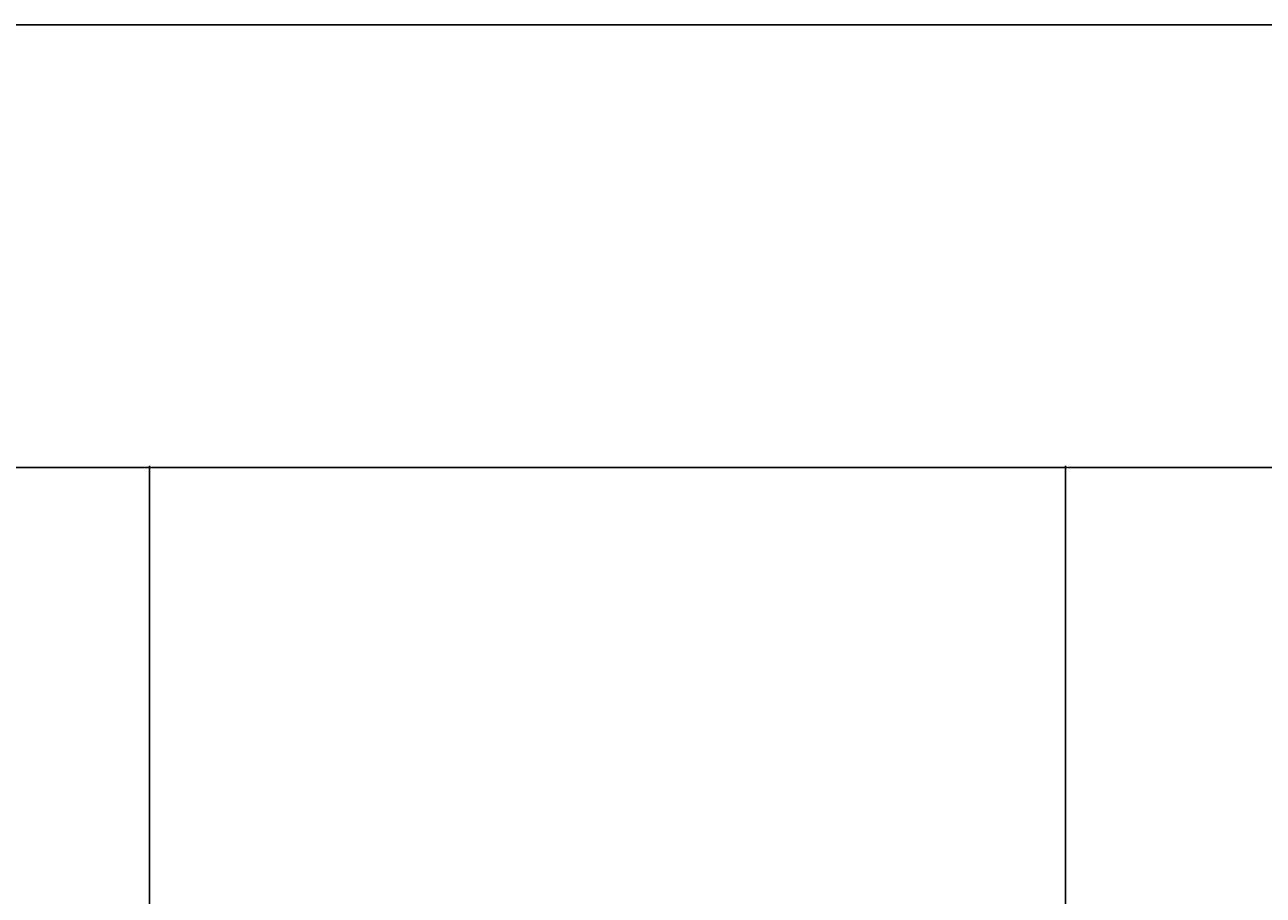
# Model space of a CAD drawing. Units: inches. Extents: x 1601 to 2297, y 1496 to 2631.
# Tile 45 of 57: x 1750 to 1891, y 2532 to 2631. Entities that reach past the tile are written whole.
import ezdxf

# ---------------------------------------------------------------- set-up
doc = ezdxf.new("R2010")
doc.units = ezdxf.units.IN
doc.layers.add('A-ANNO-DIMS', color=2, linetype='Continuous', lineweight=18)
doc.layers.add('A-ANNO-TTLB', color=7, linetype='Continuous', lineweight=25)
doc.styles.get("Standard").update_dxf_attribs({"font": 'arial.ttf'})
doc.dimstyles.get("Standard").update_dxf_attribs({"dimtxt": 0.18, "dimasz": 0.18, "dimexe": 0.18, "dimexo": 0.0625, "dimgap": 0.09, "dimtad": 0, "dimtih": 1, "dimtoh": 1, "dimdec": 4, "dimzin": 0, "dimdsep": 46, "dimtxsty": 'Standard', "dimcen": 0.09, "dimadec": 0, "dimazin": 0, "dimtfac": 1, "dimtdec": 4, "dimtofl": 0, "dimtmove": 0, "dimatfit": 3, "dimfxl": 1, "dimtolj": 1, "dimtzin": 0, "dimarcsym": 0})

# ---------------------------------------------------------------- blocks, each defined once
blk = doc.blocks.new('*D28')
at = {"layer": 'A-ANNO-DIMS', "color": 0, "lineweight": -2, "transparency": 16777216}
for p, q in [((1686.04, 2532.39), (1686.04, 2581.06)), ((1686.22, 2580.88), (1957.89, 2580.88)), ((2230.36, 2580.88), (1958.68, 2580.88)), ((2230.54, 2532.39), (2230.54, 2581.06))]:
    blk.add_line(p, q, dxfattribs=at)
at = {"layer": 'A-ANNO-DIMS', "color": 0, "transparency": 16777216}
for points in [[(1686.22, 2580.91), (1686.22, 2580.85), (1686.04, 2580.88)], [(2230.36, 2580.91), (2230.36, 2580.85), (2230.54, 2580.88)]]:
    blk.add_solid(points, dxfattribs=at)
at = {"layer": 'Defpoints', "color": 0, "transparency": 16777216}
for p in [(2230.54, 2580.88), (1686.04, 2532.33), (2230.54, 2532.33)]:
    blk.add_point(p, dxfattribs=at)
at = {"layer": 'A-ANNO-DIMS', "color": 0, "transparency": 16777216, "insert": (1958.29, 2580.88), "char_height": 0.18, "attachment_point": 5}
blk.add_mtext('\\A1;544.5', dxfattribs=at)
blk = doc.blocks.new('*D33')
at = {"layer": 'A-ANNO-DIMS', "color": 0, "lineweight": -2, "transparency": 16777216}
for p, q in [((1764.34, 2136.39), (1764.34, 2581.06)), ((1764.52, 2580.88), (1816.06, 2580.88)), ((1868.16, 2580.88), (1816.62, 2580.88)), ((1868.34, 2136.39), (1868.34, 2581.06))]:
    blk.add_line(p, q, dxfattribs=at)
at = {"layer": 'A-ANNO-DIMS', "color": 0, "transparency": 16777216}
for points in [[(1764.52, 2580.91), (1764.52, 2580.85), (1764.34, 2580.88)], [(1868.16, 2580.91), (1868.16, 2580.85), (1868.34, 2580.88)]]:
    blk.add_solid(points, dxfattribs=at)
at = {"layer": 'Defpoints', "color": 0, "transparency": 16777216}
for p in [(1868.34, 2580.88), (1764.34, 2136.33), (1868.34, 2136.33)]:
    blk.add_point(p, dxfattribs=at)
at = {"layer": 'A-ANNO-DIMS', "color": 0, "transparency": 16777216, "insert": (1816.34, 2580.88), "char_height": 0.18, "attachment_point": 5}
blk.add_mtext('\\A1;104', dxfattribs=at)

msp = doc.modelspace()

# ---------------------------------------------------------------- linework, layer by layer
at = {"layer": 'A-ANNO-TTLB'}
msp.add_lwpolyline([(1600.5933, 2631.1477), (2297.129, 2631.1477), (2297.129, 1496.1026), (1600.5933, 1496.1026)], close=True, dxfattribs=at)

# ---------------------------------------------------------------- dimensions: what is measured, and where the dimension line sits
at = {"layer": 'A-ANNO-DIMS'}
for base, p1, p2, override, picture, middle in [((2230.5373, 2580.8754), (1686.0373, 2532.3254), (2230.5373, 2532.3254), {"dimdec": 1, "dimlfac": 1, "dimrnd": 0, "dimzin": 0, "dimdsep": 46, "dimlunit": 2}, '*D28', (1958.2873, 2580.8754)), ((1868.3371, 2580.8754), (1764.3371, 2136.3254), (1868.3371, 2136.3254), {"dimdec": 0, "dimlfac": 1, "dimrnd": 0, "dimzin": 0, "dimdsep": 46, "dimlunit": 2}, '*D33', (1816.3371, 2580.8754))]:
    dim = msp.add_linear_dim(base=base, p1=p1, p2=p2, dimstyle='Standard', override=override, dxfattribs=at)
    dim.commit()
    dim.dimension.update_dxf_attribs({"geometry": picture, "text_midpoint": middle})

doc.saveas('drawing.dxf')
